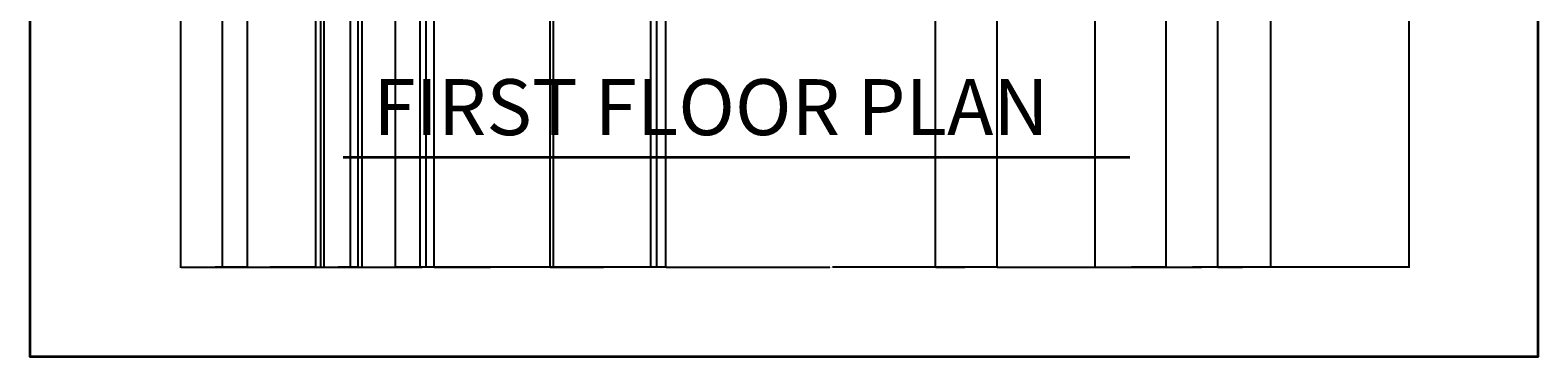
# Model space of a CAD drawing. Units: inches. Extents: x 2529 to 3014, y 1203 to 2262.
# Tile 1 of 13: x 2529 to 3014, y 1455 to 1560. Entities that reach past the tile are written whole.
import ezdxf

# ---------------------------------------------------------------- set-up
doc = ezdxf.new("R2010")
doc.units = ezdxf.units.IN
for name, color, linetype, lineweight in [('A-ANNO-DIMS', 2, 'Continuous', 18), ('A-ANNO-TITL', 21, 'Continuous', 35), ('A-ANNO-TTLB', 7, 'Continuous', 35)]:
    doc.layers.add(name, color=color, linetype=linetype, lineweight=lineweight)
doc.styles.get("Standard").update_dxf_attribs({"font": 'arial.ttf'})
doc.dimstyles.get("Standard").update_dxf_attribs({"dimtxt": 0.18, "dimasz": 0.18, "dimexe": 0.18, "dimexo": 0.0625, "dimgap": 0.09, "dimtad": 0, "dimtih": 1, "dimtoh": 1, "dimdec": 4, "dimzin": 0, "dimdsep": 46, "dimtxsty": 'Standard', "dimcen": 0.09, "dimadec": 0, "dimazin": 0, "dimtfac": 1, "dimtdec": 4, "dimtofl": 0, "dimtmove": 0, "dimatfit": 3, "dimfxl": 1, "dimtolj": 1, "dimtzin": 0, "dimarcsym": 0})

# ---------------------------------------------------------------- blocks, each defined once
blk = doc.blocks.new('*D18')
at = {"layer": 'A-ANNO-DIMS', "color": 0, "lineweight": -2, "transparency": 16777216}
for p, q in [((2577.06, 1573.44), (2577.06, 1483.77)), ((2733.06, 1573.44), (2733.06, 1483.77)), ((2577.24, 1483.95), (2654.78, 1483.95)), ((2732.88, 1483.95), (2655.34, 1483.95))]:
    blk.add_line(p, q, dxfattribs=at)
at = {"layer": 'A-ANNO-DIMS', "color": 0, "transparency": 16777216}
for points in [[(2577.24, 1483.98), (2577.24, 1483.92), (2577.06, 1483.95)], [(2732.88, 1483.98), (2732.88, 1483.92), (2733.06, 1483.95)]]:
    blk.add_solid(points, dxfattribs=at)
at = {"layer": 'Defpoints', "color": 0, "transparency": 16777216}
for p in [(2577.06, 1573.5), (2733.06, 1573.5), (2733.06, 1483.95)]:
    blk.add_point(p, dxfattribs=at)
at = {"layer": 'A-ANNO-DIMS', "color": 0, "transparency": 16777216, "insert": (2655.06, 1483.95), "char_height": 0.18, "attachment_point": 5}
blk.add_mtext('\\A1;156', dxfattribs=at)
blk = doc.blocks.new('*D19')
at = {"layer": 'A-ANNO-DIMS', "color": 0, "lineweight": -2, "transparency": 16777216}
for p, q in [((2839.56, 1582.44), (2839.56, 1483.77)), ((2733.06, 1573.44), (2733.06, 1483.77)), ((2733.24, 1483.95), (2785.92, 1483.95)), ((2839.38, 1483.95), (2786.69, 1483.95))]:
    blk.add_line(p, q, dxfattribs=at)
at = {"layer": 'A-ANNO-DIMS', "color": 0, "transparency": 16777216}
for points in [[(2733.24, 1483.98), (2733.24, 1483.92), (2733.06, 1483.95)], [(2839.38, 1483.98), (2839.38, 1483.92), (2839.56, 1483.95)]]:
    blk.add_solid(points, dxfattribs=at)
at = {"layer": 'Defpoints', "color": 0, "transparency": 16777216}
for p in [(2839.56, 1582.5), (2733.06, 1573.5), (2839.56, 1483.95)]:
    blk.add_point(p, dxfattribs=at)
at = {"layer": 'A-ANNO-DIMS', "color": 0, "transparency": 16777216, "insert": (2786.31, 1483.95), "char_height": 0.18, "attachment_point": 5}
blk.add_mtext('\\A1;106.5', dxfattribs=at)
blk = doc.blocks.new('*D20')
at = {"layer": 'A-ANNO-DIMS', "color": 0, "lineweight": -2, "transparency": 16777216}
for p, q in [((2839.56, 1582.44), (2839.56, 1483.77)), ((2972.06, 1573.44), (2972.06, 1483.77)), ((2839.74, 1483.95), (2905.42, 1483.95)), ((2971.88, 1483.95), (2906.19, 1483.95))]:
    blk.add_line(p, q, dxfattribs=at)
at = {"layer": 'A-ANNO-DIMS', "color": 0, "transparency": 16777216}
for points in [[(2839.74, 1483.98), (2839.74, 1483.92), (2839.56, 1483.95)], [(2971.88, 1483.98), (2971.88, 1483.92), (2972.06, 1483.95)]]:
    blk.add_solid(points, dxfattribs=at)
at = {"layer": 'Defpoints', "color": 0, "transparency": 16777216}
for p in [(2839.56, 1582.5), (2972.06, 1573.5), (2972.06, 1483.95)]:
    blk.add_point(p, dxfattribs=at)
at = {"layer": 'A-ANNO-DIMS', "color": 0, "transparency": 16777216, "insert": (2905.81, 1483.95), "char_height": 0.18, "attachment_point": 5}
blk.add_mtext('\\A1;132.5', dxfattribs=at)
blk = doc.blocks.new('*D33')
at = {"layer": 'A-ANNO-DIMS', "color": 0, "lineweight": -2, "transparency": 16777216}
for p, q in [((2577.06, 1603.44), (2577.06, 1483.77)), ((2598.48, 1603.44), (2598.48, 1483.77)), ((2577.24, 1483.95), (2587.37, 1483.95)), ((2598.3, 1483.95), (2588.16, 1483.95))]:
    blk.add_line(p, q, dxfattribs=at)
at = {"layer": 'A-ANNO-DIMS', "color": 0, "transparency": 16777216}
for points in [[(2577.24, 1483.98), (2577.24, 1483.92), (2577.06, 1483.95)], [(2598.3, 1483.98), (2598.3, 1483.92), (2598.48, 1483.95)]]:
    blk.add_solid(points, dxfattribs=at)
at = {"layer": 'Defpoints', "color": 0, "transparency": 16777216}
for p in [(2577.06, 1603.5), (2598.48, 1603.5), (2598.48, 1483.95)]:
    blk.add_point(p, dxfattribs=at)
at = {"layer": 'A-ANNO-DIMS', "color": 0, "transparency": 16777216, "insert": (2587.77, 1483.95), "char_height": 0.18, "attachment_point": 5}
blk.add_mtext('\\A1;21.42', dxfattribs=at)
blk = doc.blocks.new('*D34')
at = {"layer": 'A-ANNO-DIMS', "color": 0, "lineweight": -2, "transparency": 16777216}
for p, q in [((2658.48, 1603.44), (2658.48, 1483.77)), ((2695.77, 1603.44), (2695.77, 1483.77)), ((2658.66, 1483.95), (2676.73, 1483.95)), ((2695.59, 1483.95), (2677.52, 1483.95))]:
    blk.add_line(p, q, dxfattribs=at)
at = {"layer": 'A-ANNO-DIMS', "color": 0, "transparency": 16777216}
for points in [[(2658.66, 1483.98), (2658.66, 1483.92), (2658.48, 1483.95)], [(2695.59, 1483.98), (2695.59, 1483.92), (2695.77, 1483.95)]]:
    blk.add_solid(points, dxfattribs=at)
at = {"layer": 'Defpoints', "color": 0, "transparency": 16777216}
for p in [(2658.48, 1603.5), (2695.77, 1603.5), (2695.77, 1483.95)]:
    blk.add_point(p, dxfattribs=at)
at = {"layer": 'A-ANNO-DIMS', "color": 0, "transparency": 16777216, "insert": (2677.12, 1483.95), "char_height": 0.18, "attachment_point": 5}
blk.add_mtext('\\A1;37.29', dxfattribs=at)
blk = doc.blocks.new('*D35')
at = {"layer": 'A-ANNO-DIMS', "color": 0, "lineweight": -2, "transparency": 16777216}
for p, q in [((2695.77, 1603.44), (2695.77, 1483.77)), ((2728.25, 1603.44), (2728.25, 1483.77)), ((2695.95, 1483.95), (2711.61, 1483.95)), ((2728.07, 1483.95), (2712.4, 1483.95))]:
    blk.add_line(p, q, dxfattribs=at)
at = {"layer": 'A-ANNO-DIMS', "color": 0, "transparency": 16777216}
for points in [[(2695.95, 1483.98), (2695.95, 1483.92), (2695.77, 1483.95)], [(2728.07, 1483.98), (2728.07, 1483.92), (2728.25, 1483.95)]]:
    blk.add_solid(points, dxfattribs=at)
at = {"layer": 'Defpoints', "color": 0, "transparency": 16777216}
for p in [(2695.77, 1603.5), (2728.25, 1603.5), (2728.25, 1483.95)]:
    blk.add_point(p, dxfattribs=at)
at = {"layer": 'A-ANNO-DIMS', "color": 0, "transparency": 16777216, "insert": (2712.01, 1483.95), "char_height": 0.18, "attachment_point": 5}
blk.add_mtext('\\A1;32.48', dxfattribs=at)
blk = doc.blocks.new('*D41')
at = {"layer": 'A-ANNO-DIMS', "color": 0, "lineweight": -2, "transparency": 16777216}
for p, q in [((2819.79, 1733.94), (2819.79, 1483.77)), ((2839.56, 1733.94), (2839.56, 1483.77)), ((2819.97, 1483.95), (2829.29, 1483.95)), ((2839.38, 1483.95), (2830.06, 1483.95))]:
    blk.add_line(p, q, dxfattribs=at)
at = {"layer": 'A-ANNO-DIMS', "color": 0, "transparency": 16777216}
for points in [[(2819.97, 1483.98), (2819.97, 1483.92), (2819.79, 1483.95)], [(2839.38, 1483.98), (2839.38, 1483.92), (2839.56, 1483.95)]]:
    blk.add_solid(points, dxfattribs=at)
at = {"layer": 'Defpoints', "color": 0, "transparency": 16777216}
for p in [(2819.79, 1734), (2839.56, 1734), (2819.79, 1483.95)]:
    blk.add_point(p, dxfattribs=at)
at = {"layer": 'A-ANNO-DIMS', "color": 0, "transparency": 16777216, "insert": (2829.67, 1483.95), "char_height": 0.18, "attachment_point": 5}
blk.add_mtext('\\A1;19.77', dxfattribs=at)
blk = doc.blocks.new('*D42')
at = {"layer": 'A-ANNO-DIMS', "color": 0, "lineweight": -2, "transparency": 16777216}
for p, q in [((2590.48, 1640.92), (2590.48, 1483.77)), ((2620.46, 1640.92), (2620.46, 1483.77)), ((2590.66, 1483.95), (2605.07, 1483.95)), ((2620.28, 1483.95), (2605.86, 1483.95))]:
    blk.add_line(p, q, dxfattribs=at)
at = {"layer": 'A-ANNO-DIMS', "color": 0, "transparency": 16777216}
for points in [[(2590.66, 1483.98), (2590.66, 1483.92), (2590.48, 1483.95)], [(2620.28, 1483.98), (2620.28, 1483.92), (2620.46, 1483.95)]]:
    blk.add_solid(points, dxfattribs=at)
at = {"layer": 'Defpoints', "color": 0, "transparency": 16777216}
for p in [(2590.48, 1640.98), (2620.46, 1640.98), (2620.46, 1483.95)]:
    blk.add_point(p, dxfattribs=at)
at = {"layer": 'A-ANNO-DIMS', "color": 0, "transparency": 16777216, "insert": (2605.47, 1483.95), "char_height": 0.18, "attachment_point": 5}
blk.add_mtext('\\A1;29.98', dxfattribs=at)
blk = doc.blocks.new('*D44')
at = {"layer": 'A-ANNO-DIMS', "color": 0, "lineweight": -2, "transparency": 16777216}
for p, q in [((2635.37, 1678.62), (2635.37, 1483.77)), ((2655.89, 1678.62), (2655.89, 1483.77)), ((2635.55, 1483.95), (2645.17, 1483.95)), ((2655.71, 1483.95), (2646.1, 1483.95))]:
    blk.add_line(p, q, dxfattribs=at)
at = {"layer": 'A-ANNO-DIMS', "color": 0, "transparency": 16777216}
for points in [[(2635.55, 1483.98), (2635.55, 1483.92), (2635.37, 1483.95)], [(2655.71, 1483.98), (2655.71, 1483.92), (2655.89, 1483.95)]]:
    blk.add_solid(points, dxfattribs=at)
at = {"layer": 'Defpoints', "color": 0, "transparency": 16777216}
for p in [(2635.37, 1678.68), (2655.89, 1678.68), (2655.89, 1483.95)]:
    blk.add_point(p, dxfattribs=at)
at = {"layer": 'A-ANNO-DIMS', "color": 0, "transparency": 16777216, "insert": (2645.63, 1483.95), "char_height": 0.18, "attachment_point": 5}
blk.add_mtext('\\A1;20.517', dxfattribs=at)
blk = doc.blocks.new('*D53')
at = {"layer": 'A-ANNO-DIMS', "color": 0, "lineweight": -2, "transparency": 16777216}
for p, q in [((2696.93, 1790.94), (2696.93, 1483.77)), ((2730.09, 1790.94), (2730.09, 1483.77)), ((2697.11, 1483.95), (2713.11, 1483.95)), ((2729.91, 1483.95), (2713.9, 1483.95))]:
    blk.add_line(p, q, dxfattribs=at)
at = {"layer": 'A-ANNO-DIMS', "color": 0, "transparency": 16777216}
for points in [[(2697.11, 1483.98), (2697.11, 1483.92), (2696.93, 1483.95)], [(2729.91, 1483.98), (2729.91, 1483.92), (2730.09, 1483.95)]]:
    blk.add_solid(points, dxfattribs=at)
at = {"layer": 'Defpoints', "color": 0, "transparency": 16777216}
for p in [(2696.93, 1791), (2730.09, 1791), (2730.09, 1483.95)]:
    blk.add_point(p, dxfattribs=at)
at = {"layer": 'A-ANNO-DIMS', "color": 0, "transparency": 16777216, "insert": (2713.51, 1483.95), "char_height": 0.18, "attachment_point": 5}
blk.add_mtext('\\A1;33.15', dxfattribs=at)
blk = doc.blocks.new('*D57')
at = {"layer": 'A-ANNO-DIMS', "color": 0, "lineweight": -2, "transparency": 16777216}
for p, q in [((2871.06, 2198.44), (2871.06, 1483.77)), ((2893.92, 2198.44), (2893.92, 1483.77)), ((2871.24, 1483.95), (2882.02, 1483.95)), ((2893.74, 1483.95), (2882.95, 1483.95))]:
    blk.add_line(p, q, dxfattribs=at)
at = {"layer": 'A-ANNO-DIMS', "color": 0, "transparency": 16777216}
for points in [[(2871.24, 1483.98), (2871.24, 1483.92), (2871.06, 1483.95)], [(2893.74, 1483.98), (2893.74, 1483.92), (2893.92, 1483.95)]]:
    blk.add_solid(points, dxfattribs=at)
at = {"layer": 'Defpoints', "color": 0, "transparency": 16777216}
for p in [(2871.06, 2198.5), (2893.92, 2198.5), (2893.92, 1483.95)]:
    blk.add_point(p, dxfattribs=at)
at = {"layer": 'A-ANNO-DIMS', "color": 0, "transparency": 16777216, "insert": (2882.49, 1483.95), "char_height": 0.18, "attachment_point": 5}
blk.add_mtext('\\A1;22.866', dxfattribs=at)
blk = doc.blocks.new('*D65')
at = {"layer": 'A-ANNO-DIMS', "color": 0, "lineweight": -2, "transparency": 16777216}
for p, q in [((2646.06, 1874.24), (2646.06, 1483.77)), ((2654.06, 1874.24), (2654.06, 1483.77)), ((2646.24, 1483.95), (2649.91, 1483.95)), ((2653.88, 1483.95), (2650.2, 1483.95))]:
    blk.add_line(p, q, dxfattribs=at)
at = {"layer": 'A-ANNO-DIMS', "color": 0, "transparency": 16777216}
for points in [[(2646.24, 1483.98), (2646.24, 1483.92), (2646.06, 1483.95)], [(2653.88, 1483.98), (2653.88, 1483.92), (2654.06, 1483.95)]]:
    blk.add_solid(points, dxfattribs=at)
at = {"layer": 'Defpoints', "color": 0, "transparency": 16777216}
for p in [(2646.06, 1874.3), (2654.06, 1874.3), (2654.06, 1483.95)]:
    blk.add_point(p, dxfattribs=at)
at = {"layer": 'A-ANNO-DIMS', "color": 0, "transparency": 16777216, "insert": (2650.06, 1483.95), "char_height": 0.18, "attachment_point": 5}
blk.add_mtext('\\A1;8', dxfattribs=at)
blk = doc.blocks.new('*D71')
at = {"layer": 'A-ANNO-DIMS', "color": 0, "lineweight": -2, "transparency": 16777216}
for p, q in [((2623.09, 2159.68), (2623.09, 1483.77)), ((2631.58, 2159.68), (2631.58, 1483.77)), ((2623.27, 1483.95), (2626.94, 1483.95)), ((2631.4, 1483.95), (2627.73, 1483.95))]:
    blk.add_line(p, q, dxfattribs=at)
at = {"layer": 'A-ANNO-DIMS', "color": 0, "transparency": 16777216}
for points in [[(2623.27, 1483.98), (2623.27, 1483.92), (2623.09, 1483.95)], [(2631.4, 1483.98), (2631.4, 1483.92), (2631.58, 1483.95)]]:
    blk.add_solid(points, dxfattribs=at)
at = {"layer": 'Defpoints', "color": 0, "transparency": 16777216}
for p in [(2623.09, 2159.75), (2631.58, 2159.75), (2631.58, 1483.95)]:
    blk.add_point(p, dxfattribs=at)
at = {"layer": 'A-ANNO-DIMS', "color": 0, "transparency": 16777216, "insert": (2627.33, 1483.95), "char_height": 0.18, "attachment_point": 5}
blk.add_mtext('\\A1;8.484', dxfattribs=at)
blk = doc.blocks.new('*D74')
at = {"layer": 'A-ANNO-DIMS', "color": 0, "lineweight": -2, "transparency": 16777216}
for p, q in [((2622.06, 2135.91), (2622.06, 1483.77)), ((2634.06, 2135.91), (2634.06, 1483.77)), ((2622.24, 1483.95), (2627.6, 1483.95)), ((2633.88, 1483.95), (2628.51, 1483.95))]:
    blk.add_line(p, q, dxfattribs=at)
at = {"layer": 'A-ANNO-DIMS', "color": 0, "transparency": 16777216}
for points in [[(2622.24, 1483.98), (2622.24, 1483.92), (2622.06, 1483.95)], [(2633.88, 1483.98), (2633.88, 1483.92), (2634.06, 1483.95)]]:
    blk.add_solid(points, dxfattribs=at)
at = {"layer": 'Defpoints', "color": 0, "transparency": 16777216}
for p in [(2622.06, 2135.98), (2634.06, 2135.98), (2634.06, 1483.95)]:
    blk.add_point(p, dxfattribs=at)
at = {"layer": 'A-ANNO-DIMS', "color": 0, "transparency": 16777216, "insert": (2628.06, 1483.95), "char_height": 0.18, "attachment_point": 5}
blk.add_mtext('\\A1;12.002', dxfattribs=at)
blk = doc.blocks.new('*D75')
at = {"layer": 'A-ANNO-DIMS', "color": 0, "lineweight": -2, "transparency": 16777216}
for p, q in [((2893.92, 2187.06), (2893.92, 1483.77)), ((2910.52, 2189.17), (2910.52, 1483.77)), ((2894.1, 1483.95), (2901.91, 1483.95)), ((2910.34, 1483.95), (2902.54, 1483.95))]:
    blk.add_line(p, q, dxfattribs=at)
at = {"layer": 'A-ANNO-DIMS', "color": 0, "transparency": 16777216}
for points in [[(2894.1, 1483.98), (2894.1, 1483.92), (2893.92, 1483.95)], [(2910.34, 1483.98), (2910.34, 1483.92), (2910.52, 1483.95)]]:
    blk.add_solid(points, dxfattribs=at)
at = {"layer": 'Defpoints', "color": 0, "transparency": 16777216}
for p in [(2893.92, 2187.12), (2910.52, 2189.24), (2910.52, 1483.95)]:
    blk.add_point(p, dxfattribs=at)
at = {"layer": 'A-ANNO-DIMS', "color": 0, "transparency": 16777216, "insert": (2902.22, 1483.95), "char_height": 0.18, "attachment_point": 5}
blk.add_mtext('\\A1;16.6', dxfattribs=at)
blk = doc.blocks.new('*D76')
at = {"layer": 'A-ANNO-DIMS', "color": 0, "lineweight": -2, "transparency": 16777216}
for p, q in [((2910.52, 2189.17), (2910.52, 1483.77)), ((2927.64, 2189.17), (2927.64, 1483.77)), ((2910.7, 1483.95), (2918.63, 1483.95)), ((2927.46, 1483.95), (2919.54, 1483.95))]:
    blk.add_line(p, q, dxfattribs=at)
at = {"layer": 'A-ANNO-DIMS', "color": 0, "transparency": 16777216}
for points in [[(2910.7, 1483.98), (2910.7, 1483.92), (2910.52, 1483.95)], [(2927.46, 1483.98), (2927.46, 1483.92), (2927.64, 1483.95)]]:
    blk.add_solid(points, dxfattribs=at)
at = {"layer": 'Defpoints', "color": 0, "transparency": 16777216}
for p in [(2910.52, 2189.24), (2927.64, 2189.24), (2927.64, 1483.95)]:
    blk.add_point(p, dxfattribs=at)
at = {"layer": 'A-ANNO-DIMS', "color": 0, "transparency": 16777216, "insert": (2919.08, 1483.95), "char_height": 0.18, "attachment_point": 5}
blk.add_mtext('\\A1;17.123', dxfattribs=at)

msp = doc.modelspace()

# ---------------------------------------------------------------- linework, layer by layer
at = {"layer": 'A-ANNO-TITL'}
msp.add_line((2629.3873, 1519.3742), (2882.3938, 1519.3742), dxfattribs=at)
at = {"layer": 'A-ANNO-TTLB'}
msp.add_lwpolyline([(2528.6765, 2261.8165), (3013.6003, 2261.8165), (3013.6003, 1455.1523), (2528.6765, 1455.1523)], close=True, dxfattribs=at)

# ---------------------------------------------------------------- texts
at = {"layer": 'A-ANNO-TITL', "insert": (2639.0693, 1544.3953), "char_height": 18, "attachment_point": 1}
msp.add_mtext_dynamic_manual_height_columns('FIRST FLOOR PLAN ', width=333.187122, gutter_width=12.5, heights=[0], dxfattribs=at)

# ---------------------------------------------------------------- dimensions: what is measured, and where the dimension line sits
at = {"layer": 'A-ANNO-DIMS'}
for base, p1, p2, override, picture, middle in [((2893.9216, 1483.9492), (2871.0554, 2198.5032), (2893.9216, 2198.5032), {"dimdec": 3, "dimlfac": 1, "dimrnd": 0, "dimzin": 0, "dimdsep": 46, "dimlunit": 2}, '*D57', (2882.4885, 1483.9492)), ((2910.5203, 1483.9492), (2893.9216, 2187.1225), (2910.5203, 2189.237), {"dimdec": 1, "dimlfac": 1, "dimrnd": 0, "dimzin": 0, "dimdsep": 46, "dimlunit": 2}, '*D75', (2902.2209, 1483.9492)), ((2927.6434, 1483.9492), (2910.5203, 2189.237), (2927.6434, 2189.237), {"dimdec": 3, "dimlfac": 1, "dimrnd": 0, "dimzin": 0, "dimdsep": 46, "dimlunit": 2}, '*D76', (2919.0819, 1483.9492)), ((2631.5753, 1483.9492), (2623.0916, 2159.7466), (2631.5753, 2159.7466), {"dimdec": 3, "dimlfac": 1, "dimrnd": 0, "dimzin": 0, "dimdsep": 46, "dimlunit": 2}, '*D71', (2627.3335, 1483.9492)), ((2634.0572, 1483.9492), (2622.0554, 2135.9767), (2634.0572, 2135.9767), {"dimdec": 3, "dimlfac": 1, "dimrnd": 0, "dimzin": 0, "dimdsep": 46, "dimlunit": 2}, '*D74', (2628.0563, 1483.9492)), ((2654.0554, 1483.9492), (2646.0554, 1874.3024), (2654.0554, 1874.3024), {"dimdec": 0, "dimlfac": 1, "dimrnd": 0, "dimzin": 0, "dimdsep": 46, "dimlunit": 2}, '*D65', (2650.0554, 1483.9492)), ((2730.085, 1483.9492), (2696.9325, 1791.0032), (2730.085, 1791.0032), {"dimdec": 2, "dimlfac": 1, "dimrnd": 0, "dimzin": 0, "dimdsep": 46, "dimlunit": 2}, '*D53', (2713.5087, 1483.9492)), ((2819.786, 1483.9492), (2839.5554, 1734.0032), (2819.786, 1734.0032), {"dimdec": 2, "dimlfac": 1, "dimrnd": 0, "dimzin": 0, "dimdsep": 46, "dimlunit": 2}, '*D41', (2829.6707, 1483.9492)), ((2655.8904, 1483.9492), (2635.3732, 1678.6815), (2655.8904, 1678.6815), {"dimdec": 3, "dimlfac": 1, "dimrnd": 0, "dimzin": 0, "dimdsep": 46, "dimlunit": 2}, '*D44', (2645.6318, 1483.9492)), ((2620.4577, 1483.9492), (2590.4804, 1640.9787), (2620.4577, 1640.9787), {"dimdec": 2, "dimlfac": 1, "dimrnd": 0, "dimzin": 0, "dimdsep": 46, "dimlunit": 2}, '*D42', (2605.4691, 1483.9492)), ((2598.4771, 1483.9492), (2577.0554, 1603.5032), (2598.4771, 1603.5032), {"dimdec": 2, "dimlfac": 1, "dimrnd": 0, "dimzin": 0, "dimdsep": 46, "dimlunit": 2}, '*D33', (2587.7662, 1483.9492)), ((2695.7662, 1483.9492), (2658.4771, 1603.5032), (2695.7662, 1603.5032), {"dimdec": 2, "dimlfac": 1, "dimrnd": 0, "dimzin": 0, "dimdsep": 46, "dimlunit": 2}, '*D34', (2677.1217, 1483.9492)), ((2728.2475, 1483.9492), (2695.7662, 1603.5032), (2728.2475, 1603.5032), {"dimdec": 2, "dimlfac": 1, "dimrnd": 0, "dimzin": 0, "dimdsep": 46, "dimlunit": 2}, '*D35', (2712.0068, 1483.9492)), ((2839.5554, 1483.9492), (2733.0554, 1573.5032), (2839.5554, 1582.5032), {"dimdec": 1, "dimlfac": 1, "dimrnd": 0, "dimzin": 0, "dimdsep": 46, "dimlunit": 2}, '*D19', (2786.3054, 1483.9492)), ((2972.0554, 1483.9492), (2839.5554, 1582.5032), (2972.0554, 1573.5032), {"dimdec": 1, "dimlfac": 1, "dimrnd": 0, "dimzin": 0, "dimdsep": 46, "dimlunit": 2}, '*D20', (2905.8054, 1483.9492)), ((2733.0554, 1483.9492), (2577.0554, 1573.5032), (2733.0554, 1573.5032), {"dimdec": 0, "dimlfac": 1, "dimrnd": 0, "dimzin": 0, "dimdsep": 46, "dimlunit": 2}, '*D18', (2655.0554, 1483.9492))]:
    dim = msp.add_linear_dim(base=base, p1=p1, p2=p2, dimstyle='Standard', override=override, dxfattribs=at)
    dim.commit()
    dim.dimension.update_dxf_attribs({"geometry": picture, "text_midpoint": middle})

doc.saveas('drawing.dxf')
